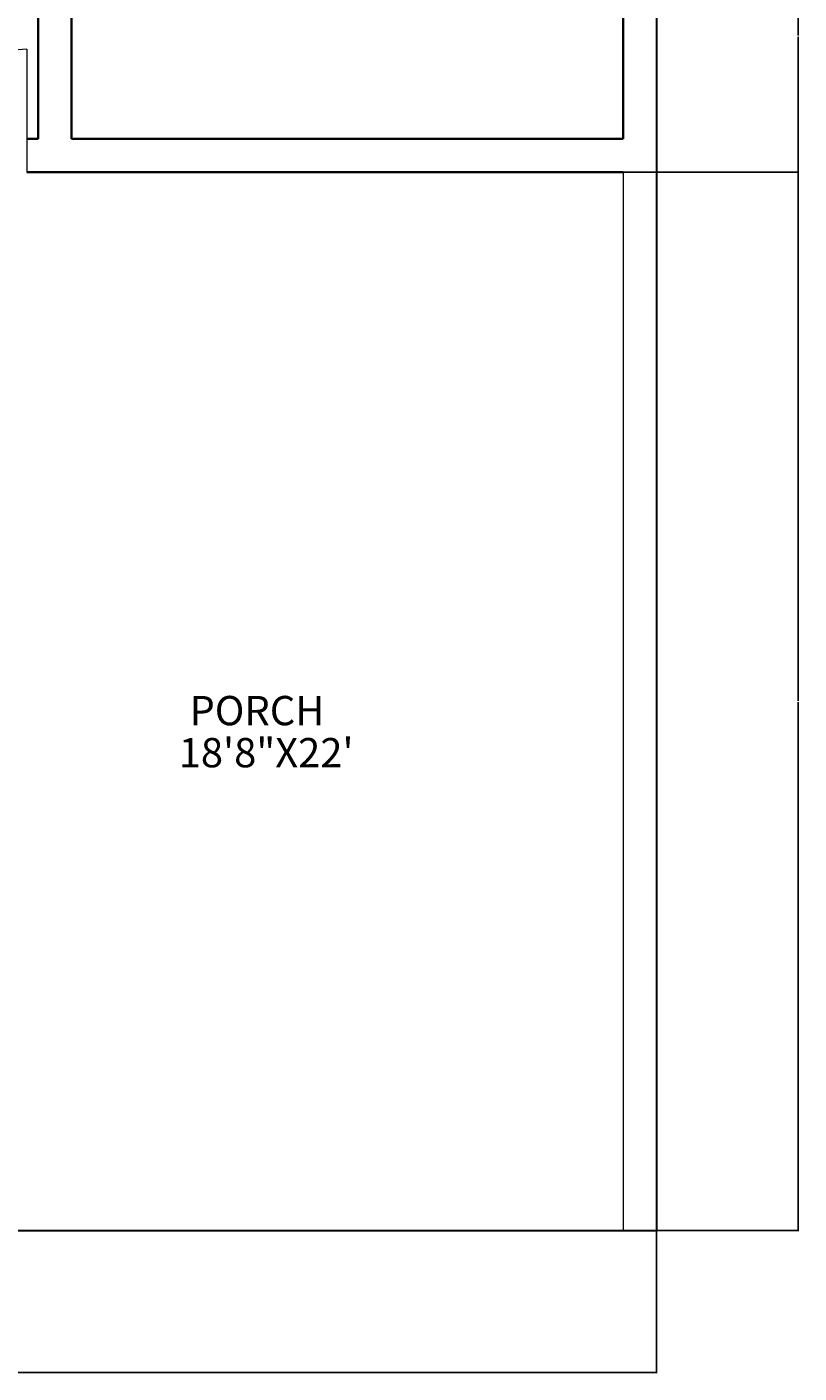
# Model space of a CAD drawing. Units: feet. Extents: x 2219 to 3039, y 1768 to 2369.
# Tile 6 of 16: x 2831 to 3039, y 1791 to 2152. Entities that reach past the tile are written whole.
import ezdxf

# ---------------------------------------------------------------- set-up
doc = ezdxf.new("R2010")
doc.units = ezdxf.units.FT
for name, color, linetype, lineweight in [('A-ANNO-DIMS', 2, 'Continuous', 18), ('A-AREA-IDEN', 7, 'Continuous', 18), ('A-DOOR', 4, 'Continuous', 20), ('A-WALL', 7, 'Continuous', 35), ('C-PROP', 7, 'Continuous', 30), ('C-SITE', 3, 'Continuous', 20)]:
    doc.layers.add(name, color=color, linetype=linetype, lineweight=lineweight)
doc.styles.get("Standard").update_dxf_attribs({"font": 'arial.ttf'})
doc.dimstyles.get("Standard").update_dxf_attribs({"dimtxt": 0.18, "dimasz": 0.18, "dimexe": 0.18, "dimexo": 0.0625, "dimgap": 0.09, "dimtad": 0, "dimtih": 1, "dimtoh": 1, "dimdec": 4, "dimzin": 0, "dimdsep": 46, "dimtxsty": 'Standard', "dimcen": 0.09, "dimadec": 0, "dimazin": 0, "dimtfac": 1, "dimtdec": 4, "dimtofl": 0, "dimtmove": 0, "dimatfit": 3, "dimfxl": 1, "dimtolj": 1, "dimtzin": 0, "dimarcsym": 0})

# ---------------------------------------------------------------- blocks, each defined once
blk = doc.blocks.new('DOOR-24-LEAF')
blk.add_line((33, 0), (0, 0))
blk.add_arc((9, 0), 24, 0, 90)
blk = doc.blocks.new('*D46')
at = {"layer": 'A-ANNO-DIMS', "color": 0, "lineweight": -2, "transparency": 16777216}
for p, q in [((2257.4, 1828.86), (2257.4, 1790.69)), ((3000.4, 1828.86), (3000.4, 1790.69)), ((2257.58, 1790.87), (2628.61, 1790.87)), ((3000.22, 1790.87), (2629.19, 1790.87))]:
    blk.add_line(p, q, dxfattribs=at)
at = {"layer": 'A-ANNO-DIMS', "color": 0, "transparency": 16777216}
for points in [[(2257.58, 1790.9), (2257.58, 1790.84), (2257.4, 1790.87)], [(3000.22, 1790.9), (3000.22, 1790.84), (3000.4, 1790.87)]]:
    blk.add_solid(points, dxfattribs=at)
at = {"layer": 'Defpoints', "color": 0, "transparency": 16777216}
for p in [(2257.4, 1828.92), (3000.4, 1828.92), (3000.4, 1790.87)]:
    blk.add_point(p, dxfattribs=at)
at = {"layer": 'A-ANNO-DIMS', "color": 0, "transparency": 16777216, "insert": (2628.9, 1790.87), "char_height": 0.18, "attachment_point": 5}
blk.add_mtext('\\A1;743', dxfattribs=at)
blk = doc.blocks.new('*D49')
at = {"layer": 'A-ANNO-DIMS', "color": 0, "lineweight": -2, "transparency": 16777216}
for p, q in [((2991.46, 2112.92), (3038.63, 2112.92)), ((3038.45, 2112.74), (3038.45, 1971.1)), ((3038.45, 1829.1), (3038.45, 1970.74)), ((3000.46, 1828.92), (3038.63, 1828.92))]:
    blk.add_line(p, q, dxfattribs=at)
at = {"layer": 'A-ANNO-DIMS', "color": 0, "transparency": 16777216}
for points in [[(3038.42, 2112.74), (3038.48, 2112.74), (3038.45, 2112.92)], [(3038.42, 1829.1), (3038.48, 1829.1), (3038.45, 1828.92)]]:
    blk.add_solid(points, dxfattribs=at)
at = {"layer": 'Defpoints', "color": 0, "transparency": 16777216}
for p in [(2991.4, 2112.92), (3038.45, 2112.92), (3000.4, 1828.92)]:
    blk.add_point(p, dxfattribs=at)
at = {"layer": 'A-ANNO-DIMS', "color": 0, "transparency": 16777216, "insert": (3038.45, 1970.92), "char_height": 0.18, "attachment_point": 5}
blk.add_mtext('\\A1;284', dxfattribs=at)
blk = doc.blocks.new('*D50')
at = {"layer": 'A-ANNO-DIMS', "color": 0, "lineweight": -2, "transparency": 16777216}
for p, q in [((3000.46, 2185.92), (3038.63, 2185.92)), ((3038.45, 2185.74), (3038.45, 2149.6)), ((3038.45, 2113.1), (3038.45, 2149.24)), ((2991.46, 2112.92), (3038.63, 2112.92))]:
    blk.add_line(p, q, dxfattribs=at)
at = {"layer": 'A-ANNO-DIMS', "color": 0, "transparency": 16777216}
for points in [[(3038.42, 2185.74), (3038.48, 2185.74), (3038.45, 2185.92)], [(3038.42, 2113.1), (3038.48, 2113.1), (3038.45, 2112.92)]]:
    blk.add_solid(points, dxfattribs=at)
at = {"layer": 'Defpoints', "color": 0, "transparency": 16777216}
for p in [(3000.4, 2185.92), (3038.45, 2185.92), (2991.4, 2112.92)]:
    blk.add_point(p, dxfattribs=at)
at = {"layer": 'A-ANNO-DIMS', "color": 0, "transparency": 16777216, "insert": (3038.45, 2149.42), "char_height": 0.18, "attachment_point": 5}
blk.add_mtext('\\A1;73', dxfattribs=at)

msp = doc.modelspace()

# ---------------------------------------------------------------- linework, layer by layer
at = {"layer": 'A-WALL'}
for p, q in [((2991.4, 2321.923), (2991.4, 2121.923)), ((2834.4, 2180.687), (2834.4, 2121.923)), ((2843.4, 2180.687), (2843.4, 2121.923)), ((2834.4, 2121.923), (2831.4, 2121.923)), ((2991.4, 2121.923), (2843.4, 2121.923)), ((2991.4, 2112.923), (2831.4, 2112.923))]:
    msp.add_line(p, q, dxfattribs=at)
at = {"layer": 'C-PROP'}
for p in [(3000.4, 2330.923), (2314.4, 1828.923)]:
    msp.add_line(p, (3000.4, 1828.923), dxfattribs=at)
at = {"layer": 'C-SITE'}
msp.add_line((2991.4, 2112.923), (2991.4, 1828.923), dxfattribs=at)

# ---------------------------------------------------------------- block references
at = {"layer": 'A-DOOR', "rotation": 89.99999999999905}
msp.add_blockref('DOOR-24-LEAF', (2831.399, 2112.923), dxfattribs=at)

# ---------------------------------------------------------------- texts
at = {"layer": 'A-AREA-IDEN'}
for s, p in [('PORCH', (2875.04, 1964.54)), ('18\'8"X22\'', (2872.138, 1953.254))]:
    msp.add_text(s, height=7.8584, dxfattribs=at).set_placement(p)

# ---------------------------------------------------------------- dimensions: what is measured, and where the dimension line sits
at = {"layer": 'A-ANNO-DIMS'}
for base, p1, p2, picture, middle in [((3038.45, 2185.923), (2991.4, 2112.923), (3000.4, 2185.923), '*D50', (3038.45, 2149.423)), ((3038.45, 2112.923), (3000.4, 1828.923), (2991.4, 2112.923), '*D49', (3038.45, 1970.923))]:
    dim = msp.add_linear_dim(base=base, p1=p1, p2=p2, angle=90, dimstyle='Standard', override={"dimdec": 0, "dimlfac": 1, "dimrnd": 0, "dimzin": 0, "dimdsep": 46, "dimlunit": 2}, dxfattribs=at)
    dim.commit()
    dim.dimension.update_dxf_attribs({"geometry": picture, "text_midpoint": middle})
dim = msp.add_linear_dim(base=(3000.4, 1790.873), p1=(2257.4, 1828.923), p2=(3000.4, 1828.923), dimstyle='Standard', override={"dimdec": 0, "dimlfac": 1, "dimrnd": 0, "dimzin": 0, "dimdsep": 46, "dimlunit": 2}, dxfattribs=at)
dim.commit()
dim.dimension.update_dxf_attribs({"geometry": '*D46', "text_midpoint": (2628.9, 1790.873)})

doc.saveas('drawing.dxf')
